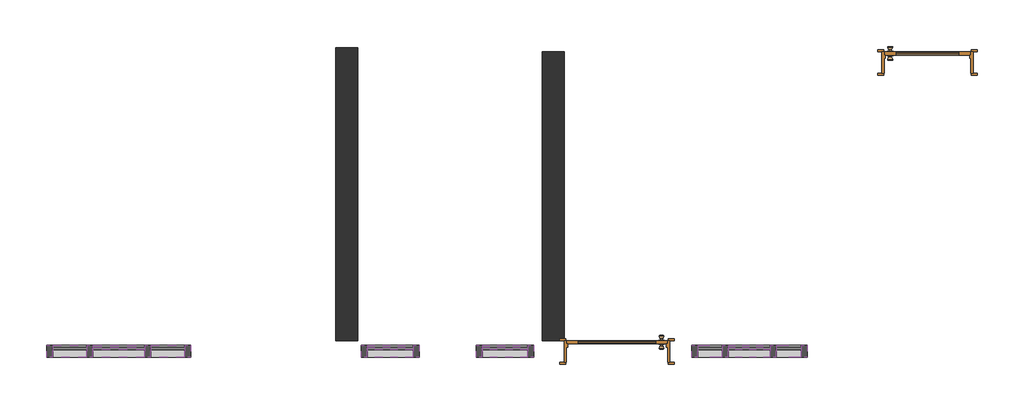
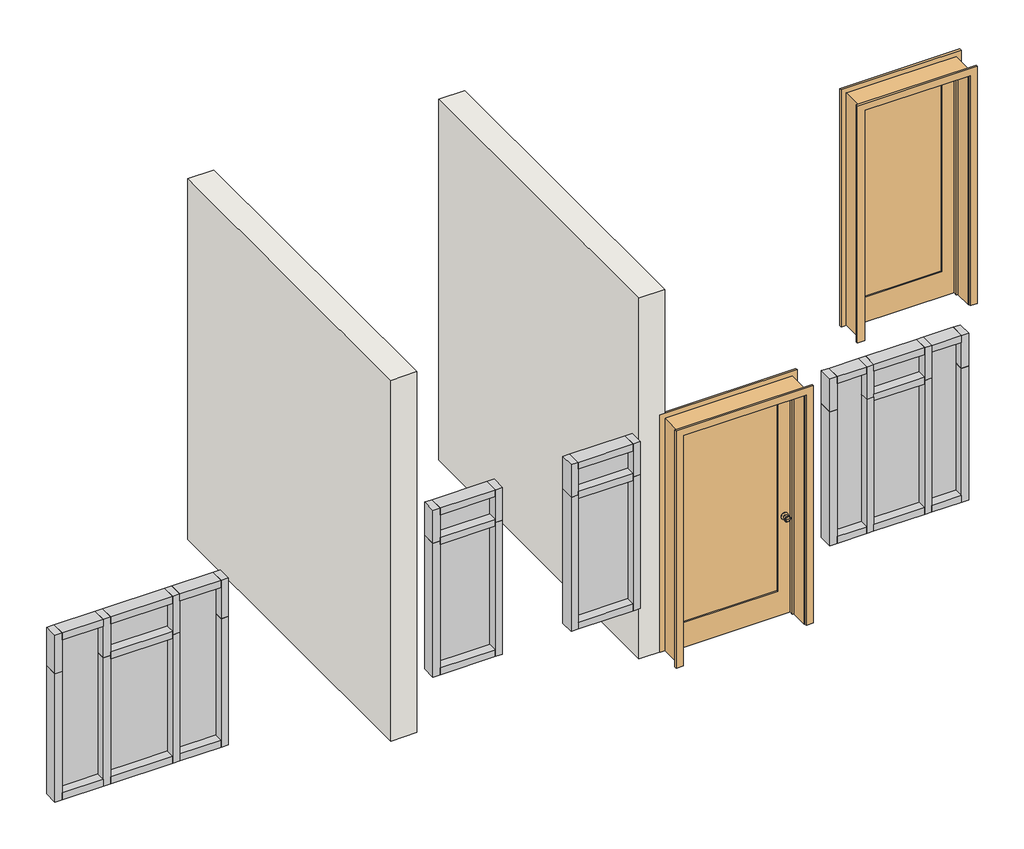
# One storey: 44 members, 12 plates, 2 doors, 2 walls.
"""IFC4 building model written with IfcOpenShell, lengths in millimetres."""

from ifc_helpers import new_model, si_unit, frame, origin, place, context, project, spatial, polyline, outline, extrude, faceted_brep, transform, mapped, element, save
from components import door_interior_single_1_panel_wood_3_x_7_3b97b8e7, door_0f538abb, member_86d06fe4, member_323df77c, member_71eb4692, member_843225dc, member_2d647432, member_0a1a1ade, member_a980948f, member_83167d3d, member_3c3dc66a, member_ca359333, member_ffcd2ccf, member_4adcbd6e, member_bc7dbe04, member_a1da5be3, member_718fe5d9, member_75d1e245, system_panel_glazed_030ff9b4, system_panel_glazed_82984963, system_panel_glazed_5eb04348, system_panel_glazed_05e747e2, system_panel_glazed_6bbf35ba, system_panel_glazed_1627a9b9, system_panel_glazed_6ade1748, system_panel_glazed_28683af0, system_panel_glazed_ad29da2a, system_panel_glazed_c196d27b

model = new_model("IFC4")

# Units and contexts
model_context = context("Model", 3, world=origin())
ifc_project = project(units=[si_unit("LENGTHUNIT", "METRE", prefix="MILLI")], contexts=[model_context])

# Site, building, storey
site = spatial("IfcSite", under=ifc_project)
building = spatial("IfcBuilding", under=site)
storey = spatial("IfcBuildingStorey", under=building, Elevation=609.6)

# Doors
placement = place(None, origin())
door_interior_single_1_panel_wood_3_x_7_shape = door_interior_single_1_panel_wood_3_x_7_3b97b8e7(model_context)
element("IfcDoor", 1, ObjectType="Door-Interior-Single-1_Panel-Wood : 3' x 7'", at=placement, inside=storey, context=model_context, shape_type="MappedRepresentation", body=[
    mapped(door_interior_single_1_panel_wood_3_x_7_shape, transform((6369.2850465, 1686.8408196, 609.6), x_axis=(1.0, 0.0, 0.0), y_axis=(0.0, 1.0, 0.0), z_axis=(0.0, 0.0, 1.0))),
])
door_shape = door_0f538abb(model_context)
element("IfcDoor", 2, ObjectType="Door-Interior-Single-1_Panel-Wood : 3'6\" x 7' DOOR", at=placement, inside=storey, context=model_context, shape_type="MappedRepresentation", body=[
    mapped(door_shape, transform((3092.6850465, -1361.1591804, 609.6), x_axis=(-1.0, 0.0, 0.0), y_axis=(0.0, -1.0, 0.0), z_axis=(0.0, 0.0, 1.0))),
])

# Members
member_shape = member_86d06fe4(model_context)
element("IfcMember", 3, ObjectType="Rectangular Mullion : 2.5\" x 5\" rectangular", at=placement, inside=storey, context=model_context, shape_type="MappedRepresentation", body=[
    mapped(member_shape, transform((940.0350465, -1364.3341804, 2768.6), x_axis=(0.0, 0.0, 1.0), y_axis=(0.0, -1.0, 0.0), z_axis=(1.0, 0.0, 0.0))),
])
element("IfcMember", 4, ObjectType="Rectangular Mullion : 2.5\" x 5\" rectangular", at=placement, inside=storey, context=model_context, shape_type="MappedRepresentation", body=[
    mapped(member_shape, transform((457.4350465, -1364.3341804, 1219.2), x_axis=(0.0, 0.0, -1.0), y_axis=(0.0, -1.0, 0.0), z_axis=(-1.0, 0.0, 0.0))),
])
member_2_shape = member_323df77c(model_context)
element("IfcMember", 5, ObjectType="Rectangular Mullion : 2.5\" x 5\" rectangular", at=placement, inside=storey, context=model_context, shape_type="MappedRepresentation", body=[
    mapped(member_2_shape, transform((940.0350465, -1364.3341804, 2463.8), x_axis=(0.0, 0.0, 1.0), y_axis=(0.0, -1.0, 0.0), z_axis=(1.0, 0.0, 0.0))),
])
member_3_shape = member_71eb4692(model_context)
element("IfcMember", 6, ObjectType="Rectangular Mullion : 2.5\" x 5\" rectangular", at=placement, inside=storey, context=model_context, shape_type="MappedRepresentation", body=[
    mapped(member_3_shape, transform((1003.5350465, -1364.3341804, 1219.2), x_axis=(1.0, 0.0, 0.0), y_axis=(0.0, -1.0, 0.0), z_axis=(0.0, 0.0, -1.0))),
])
element("IfcMember", 7, ObjectType="Rectangular Mullion : 2.5\" x 5\" rectangular", at=placement, inside=storey, context=model_context, shape_type="MappedRepresentation", body=[
    mapped(member_3_shape, transform((393.9350465, -1364.3341804, 2463.8), x_axis=(-1.0, 0.0, 0.0), y_axis=(0.0, -1.0, 0.0), z_axis=(0.0, 0.0, 1.0))),
])
element("IfcMember", 8, ObjectType="Rectangular Mullion : 2.5\" x 5\" rectangular", at=placement, inside=storey, context=model_context, shape_type="MappedRepresentation", body=[
    mapped(member_shape, transform((1670.2850465, -1364.3341804, 2768.6), x_axis=(0.0, 0.0, 1.0), y_axis=(0.0, 1.0, 0.0), z_axis=(-1.0, 0.0, 0.0))),
])
element("IfcMember", 9, ObjectType="Rectangular Mullion : 2.5\" x 5\" rectangular", at=placement, inside=storey, context=model_context, shape_type="MappedRepresentation", body=[
    mapped(member_shape, transform((2152.8850465, -1364.3341804, 1219.2), x_axis=(0.0, 0.0, -1.0), y_axis=(0.0, 1.0, 0.0), z_axis=(1.0, 0.0, 0.0))),
])
element("IfcMember", 10, ObjectType="Rectangular Mullion : 2.5\" x 5\" rectangular", at=placement, inside=storey, context=model_context, shape_type="MappedRepresentation", body=[
    mapped(member_2_shape, transform((1670.2850465, -1364.3341804, 2463.8), x_axis=(0.0, 0.0, 1.0), y_axis=(0.0, 1.0, 0.0), z_axis=(-1.0, 0.0, 0.0))),
])
element("IfcMember", 11, ObjectType="Rectangular Mullion : 2.5\" x 5\" rectangular", at=placement, inside=storey, context=model_context, shape_type="MappedRepresentation", body=[
    mapped(member_3_shape, transform((1606.7850465, -1364.3341804, 1219.2), x_axis=(-1.0, 0.0, 0.0), y_axis=(0.0, 1.0, 0.0), z_axis=(0.0, 0.0, -1.0))),
])
element("IfcMember", 12, ObjectType="Rectangular Mullion : 2.5\" x 5\" rectangular", at=placement, inside=storey, context=model_context, shape_type="MappedRepresentation", body=[
    mapped(member_3_shape, transform((2216.3850465, -1364.3341804, 2463.8), x_axis=(1.0, 0.0, 0.0), y_axis=(0.0, 1.0, 0.0), z_axis=(0.0, 0.0, 1.0))),
])
member_4_shape = member_843225dc(model_context)
element("IfcMember", 13, ObjectType="Rectangular Mullion : 2.5\" x 5\" rectangular", at=placement, inside=storey, context=model_context, shape_type="MappedRepresentation", body=[
    mapped(member_4_shape, transform((-1466.6149535, -1364.3341804, 2768.6), x_axis=(0.0, 0.0, 1.0), y_axis=(0.0, -1.0, 0.0), z_axis=(1.0, 0.0, 0.0))),
])
element("IfcMember", 14, ObjectType="Rectangular Mullion : 2.5\" x 5\" rectangular", at=placement, inside=storey, context=model_context, shape_type="MappedRepresentation", body=[
    mapped(member_4_shape, transform((-2501.6649535, -1364.3341804, 2768.6), x_axis=(0.0, 0.0, 1.0), y_axis=(0.0, -1.0, 0.0), z_axis=(1.0, 0.0, 0.0))),
])
element("IfcMember", 15, ObjectType="Rectangular Mullion : 2.5\" x 5\" rectangular", at=placement, inside=storey, context=model_context, shape_type="MappedRepresentation", body=[
    mapped(member_4_shape, transform((-2863.6149535, -1364.3341804, 1219.2), x_axis=(0.0, 0.0, -1.0), y_axis=(0.0, -1.0, 0.0), z_axis=(-1.0, 0.0, 0.0))),
])
element("IfcMember", 16, ObjectType="Rectangular Mullion : 2.5\" x 5\" rectangular", at=placement, inside=storey, context=model_context, shape_type="MappedRepresentation", body=[
    mapped(member_4_shape, transform((-1828.5649535, -1364.3341804, 1219.2), x_axis=(0.0, 0.0, -1.0), y_axis=(0.0, -1.0, 0.0), z_axis=(-1.0, 0.0, 0.0))),
])
member_5_shape = member_2d647432(model_context)
element("IfcMember", 17, ObjectType="Rectangular Mullion : 2.5\" x 5\" rectangular", at=placement, inside=storey, context=model_context, shape_type="MappedRepresentation", body=[
    mapped(member_5_shape, transform((-2469.9149535, -1364.3341804, 1219.2), x_axis=(1.0, 0.0, 0.0), y_axis=(0.0, -1.0, 0.0), z_axis=(0.0, 0.0, -1.0))),
])
element("IfcMember", 18, ObjectType="Rectangular Mullion : 2.5\" x 5\" rectangular", at=placement, inside=storey, context=model_context, shape_type="MappedRepresentation", body=[
    mapped(member_5_shape, transform((-1860.3149535, -1364.3341804, 1219.2), x_axis=(1.0, 0.0, 0.0), y_axis=(0.0, -1.0, 0.0), z_axis=(0.0, 0.0, -1.0))),
])
member_6_shape = member_0a1a1ade(model_context)
element("IfcMember", 19, ObjectType="Rectangular Mullion : 2.5\" x 5\" rectangular", at=placement, inside=storey, context=model_context, shape_type="MappedRepresentation", body=[
    mapped(member_6_shape, transform((-1892.0649535, -1364.3341804, 2413.0), x_axis=(0.0, 0.0, 1.0), y_axis=(0.0, -1.0, 0.0), z_axis=(1.0, 0.0, 0.0))),
])
member_7_shape = member_a980948f(model_context)
element("IfcMember", 20, ObjectType="Rectangular Mullion : 2.5\" x 5\" rectangular", at=placement, inside=storey, context=model_context, shape_type="MappedRepresentation", body=[
    mapped(member_7_shape, transform((-2438.1649535, -1364.3341804, 1219.2), x_axis=(0.0, 0.0, -1.0), y_axis=(0.0, -1.0, 0.0), z_axis=(-1.0, 0.0, 0.0))),
])
element("IfcMember", 21, ObjectType="Rectangular Mullion : 2.5\" x 5\" rectangular", at=placement, inside=storey, context=model_context, shape_type="MappedRepresentation", body=[
    mapped(member_7_shape, transform((-1892.0649535, -1364.3341804, 2768.6), x_axis=(0.0, 0.0, 1.0), y_axis=(0.0, -1.0, 0.0), z_axis=(1.0, 0.0, 0.0))),
])
member_8_shape = member_83167d3d(model_context)
element("IfcMember", 22, ObjectType="Rectangular Mullion : 2.5\" x 5\" rectangular", at=placement, inside=storey, context=model_context, shape_type="MappedRepresentation", body=[
    mapped(member_8_shape, transform((-1403.1149535, -1364.3341804, 1219.2), x_axis=(1.0, 0.0, 0.0), y_axis=(0.0, -1.0, 0.0), z_axis=(0.0, 0.0, -1.0))),
])
element("IfcMember", 23, ObjectType="Rectangular Mullion : 2.5\" x 5\" rectangular", at=placement, inside=storey, context=model_context, shape_type="MappedRepresentation", body=[
    mapped(member_8_shape, transform((-2927.1149535, -1364.3341804, 2413.0), x_axis=(-1.0, 0.0, 0.0), y_axis=(0.0, -1.0, 0.0), z_axis=(0.0, 0.0, 1.0))),
])
member_9_shape = member_3c3dc66a(model_context)
element("IfcMember", 24, ObjectType="Rectangular Mullion : 2.5\" x 5\" rectangular", at=placement, inside=storey, context=model_context, shape_type="MappedRepresentation", body=[
    mapped(member_9_shape, transform((2216.3850465, -1364.3341804, 2768.6), x_axis=(1.0, 0.0, 0.0), y_axis=(0.0, 1.0, 0.0), z_axis=(0.0, 0.0, 1.0))),
])
element("IfcMember", 25, ObjectType="Rectangular Mullion : 2.5\" x 5\" rectangular", at=placement, inside=storey, context=model_context, shape_type="MappedRepresentation", body=[
    mapped(member_9_shape, transform((1606.7850465, -1364.3341804, 2463.8), x_axis=(-1.0, 0.0, 0.0), y_axis=(0.0, 1.0, 0.0), z_axis=(0.0, 0.0, -1.0))),
])
element("IfcMember", 26, ObjectType="Rectangular Mullion : 2.5\" x 5\" rectangular", at=placement, inside=storey, context=model_context, shape_type="MappedRepresentation", body=[
    mapped(member_9_shape, transform((393.9350465, -1364.3341804, 2768.6), x_axis=(-1.0, 0.0, 0.0), y_axis=(0.0, -1.0, 0.0), z_axis=(0.0, 0.0, 1.0))),
])
element("IfcMember", 27, ObjectType="Rectangular Mullion : 2.5\" x 5\" rectangular", at=placement, inside=storey, context=model_context, shape_type="MappedRepresentation", body=[
    mapped(member_9_shape, transform((1003.5350465, -1364.3341804, 2463.8), x_axis=(1.0, 0.0, 0.0), y_axis=(0.0, -1.0, 0.0), z_axis=(0.0, 0.0, -1.0))),
])
member_10_shape = member_ca359333(model_context)
element("IfcMember", 28, ObjectType="Rectangular Mullion : 2.5\" x 5\" rectangular", at=placement, inside=storey, context=model_context, shape_type="MappedRepresentation", body=[
    mapped(member_10_shape, transform((-2469.9149535, -1364.3341804, 2413.0), x_axis=(1.0, 0.0, 0.0), y_axis=(0.0, -1.0, 0.0), z_axis=(0.0, 0.0, -1.0))),
])
element("IfcMember", 29, ObjectType="Rectangular Mullion : 2.5\" x 5\" rectangular", at=placement, inside=storey, context=model_context, shape_type="MappedRepresentation", body=[
    mapped(member_10_shape, transform((-1860.3149535, -1364.3341804, 2413.0), x_axis=(1.0, 0.0, 0.0), y_axis=(0.0, -1.0, 0.0), z_axis=(0.0, 0.0, -1.0))),
])
member_11_shape = member_ffcd2ccf(model_context)
element("IfcMember", 30, ObjectType="Rectangular Mullion : 2.5\" x 5\" rectangular", at=placement, inside=storey, context=model_context, shape_type="MappedRepresentation", body=[
    mapped(member_11_shape, transform((-2927.1149535, -1364.3341804, 2768.6), x_axis=(-1.0, 0.0, 0.0), y_axis=(0.0, -1.0, 0.0), z_axis=(0.0, 0.0, 1.0))),
])
element("IfcMember", 31, ObjectType="Rectangular Mullion : 2.5\" x 5\" rectangular", at=placement, inside=storey, context=model_context, shape_type="MappedRepresentation", body=[
    mapped(member_11_shape, transform((-1403.1149535, -1364.3341804, 2413.0), x_axis=(1.0, 0.0, 0.0), y_axis=(0.0, -1.0, 0.0), z_axis=(0.0, 0.0, -1.0))),
])
element("IfcMember", 32, ObjectType="Rectangular Mullion : 2.5\" x 5\" rectangular", at=placement, inside=storey, context=model_context, shape_type="MappedRepresentation", body=[
    mapped(member_9_shape, transform((3880.0850465, -1364.3341804, 2768.6), x_axis=(-1.0, 0.0, 0.0), y_axis=(0.0, -1.0, 0.0), z_axis=(0.0, 0.0, 1.0))),
])
element("IfcMember", 33, ObjectType="Rectangular Mullion : 2.5\" x 5\" rectangular", at=placement, inside=storey, context=model_context, shape_type="MappedRepresentation", body=[
    mapped(member_3_shape, transform((5099.2850465, -1364.3341804, 1219.2), x_axis=(1.0, 0.0, 0.0), y_axis=(0.0, -1.0, 0.0), z_axis=(0.0, 0.0, -1.0))),
])
element("IfcMember", 34, ObjectType="Rectangular Mullion : 2.5\" x 5\" rectangular", at=placement, inside=storey, context=model_context, shape_type="MappedRepresentation", body=[
    mapped(member_9_shape, transform((5099.2850465, -1364.3341804, 2463.8), x_axis=(1.0, 0.0, 0.0), y_axis=(0.0, -1.0, 0.0), z_axis=(0.0, 0.0, -1.0))),
])
element("IfcMember", 35, ObjectType="Rectangular Mullion : 2.5\" x 5\" rectangular", at=placement, inside=storey, context=model_context, shape_type="MappedRepresentation", body=[
    mapped(member_3_shape, transform((3880.0850465, -1364.3341804, 2463.8), x_axis=(-1.0, 0.0, 0.0), y_axis=(0.0, -1.0, 0.0), z_axis=(0.0, 0.0, 1.0))),
])
member_12_shape = member_4adcbd6e(model_context)
element("IfcMember", 36, ObjectType="Rectangular Mullion : 2.5\" x 5\" rectangular", at=placement, inside=storey, context=model_context, shape_type="MappedRepresentation", body=[
    mapped(member_12_shape, transform((5035.7850465, -1364.3341804, 2768.6), x_axis=(0.0, 0.0, 1.0), y_axis=(0.0, -1.0, 0.0), z_axis=(1.0, 0.0, 0.0))),
])
element("IfcMember", 37, ObjectType="Rectangular Mullion : 2.5\" x 5\" rectangular", at=placement, inside=storey, context=model_context, shape_type="MappedRepresentation", body=[
    mapped(member_12_shape, transform((4203.9350465, -1364.3341804, 2768.6), x_axis=(0.0, 0.0, 1.0), y_axis=(0.0, -1.0, 0.0), z_axis=(1.0, 0.0, 0.0))),
])
element("IfcMember", 38, ObjectType="Rectangular Mullion : 2.5\" x 5\" rectangular", at=placement, inside=storey, context=model_context, shape_type="MappedRepresentation", body=[
    mapped(member_12_shape, transform((3943.5850465, -1364.3341804, 1219.2), x_axis=(0.0, 0.0, -1.0), y_axis=(0.0, -1.0, 0.0), z_axis=(-1.0, 0.0, 0.0))),
])
element("IfcMember", 39, ObjectType="Rectangular Mullion : 2.5\" x 5\" rectangular", at=placement, inside=storey, context=model_context, shape_type="MappedRepresentation", body=[
    mapped(member_12_shape, transform((4775.4350465, -1364.3341804, 1219.2), x_axis=(0.0, 0.0, -1.0), y_axis=(0.0, -1.0, 0.0), z_axis=(-1.0, 0.0, 0.0))),
])
member_13_shape = member_bc7dbe04(model_context)
element("IfcMember", 40, ObjectType="Rectangular Mullion : 2.5\" x 5\" rectangular", at=placement, inside=storey, context=model_context, shape_type="MappedRepresentation", body=[
    mapped(member_13_shape, transform((4267.4350465, -1364.3341804, 1219.2), x_axis=(0.0, 0.0, -1.0), y_axis=(0.0, -1.0, 0.0), z_axis=(-1.0, 0.0, 0.0))),
])
element("IfcMember", 41, ObjectType="Rectangular Mullion : 2.5\" x 5\" rectangular", at=placement, inside=storey, context=model_context, shape_type="MappedRepresentation", body=[
    mapped(member_13_shape, transform((4711.9350465, -1364.3341804, 2768.6), x_axis=(0.0, 0.0, 1.0), y_axis=(0.0, -1.0, 0.0), z_axis=(1.0, 0.0, 0.0))),
])
member_14_shape = member_a1da5be3(model_context)
element("IfcMember", 42, ObjectType="Rectangular Mullion : 2.5\" x 5\" rectangular", at=placement, inside=storey, context=model_context, shape_type="MappedRepresentation", body=[
    mapped(member_14_shape, transform((4235.6850465, -1364.3341804, 1219.2), x_axis=(1.0, 0.0, 0.0), y_axis=(0.0, -1.0, 0.0), z_axis=(0.0, 0.0, -1.0))),
])
element("IfcMember", 43, ObjectType="Rectangular Mullion : 2.5\" x 5\" rectangular", at=placement, inside=storey, context=model_context, shape_type="MappedRepresentation", body=[
    mapped(member_14_shape, transform((4743.6850465, -1364.3341804, 1219.2), x_axis=(1.0, 0.0, 0.0), y_axis=(0.0, -1.0, 0.0), z_axis=(0.0, 0.0, -1.0))),
])
member_15_shape = member_718fe5d9(model_context)
element("IfcMember", 44, ObjectType="Rectangular Mullion : 2.5\" x 5\" rectangular", at=placement, inside=storey, context=model_context, shape_type="MappedRepresentation", body=[
    mapped(member_15_shape, transform((4711.9350465, -1364.3341804, 2463.8), x_axis=(0.0, 0.0, 1.0), y_axis=(0.0, -1.0, 0.0), z_axis=(1.0, 0.0, 0.0))),
])
member_16_shape = member_75d1e245(model_context)
element("IfcMember", 45, ObjectType="Rectangular Mullion : 2.5\" x 5\" rectangular", at=placement, inside=storey, context=model_context, shape_type="MappedRepresentation", body=[
    mapped(member_16_shape, transform((4235.6850465, -1364.3341804, 2463.8), x_axis=(1.0, 0.0, 0.0), y_axis=(0.0, -1.0, 0.0), z_axis=(0.0, 0.0, -1.0))),
])
element("IfcMember", 46, ObjectType="Rectangular Mullion : 2.5\" x 5\" rectangular", at=placement, inside=storey, context=model_context, shape_type="MappedRepresentation", body=[
    mapped(member_16_shape, transform((4743.6850465, -1364.3341804, 2463.8), x_axis=(1.0, 0.0, 0.0), y_axis=(0.0, -1.0, 0.0), z_axis=(0.0, 0.0, -1.0))),
])

# Plates
system_panel_glazed_shape = system_panel_glazed_030ff9b4(model_context)
element("IfcPlate", 47, ObjectType="System Panel : Glazed", at=placement, inside=storey, context=model_context, shape_type="MappedRepresentation", body=[
    mapped(system_panel_glazed_shape, transform((698.7350465, -1364.3341804, 1282.7), x_axis=(1.0, 0.0, 0.0), y_axis=(0.0, 1.0, 0.0), z_axis=(0.0, 0.0, 1.0))),
])
system_panel_glazed_2_shape = system_panel_glazed_82984963(model_context)
element("IfcPlate", 48, ObjectType="System Panel : Glazed", at=placement, inside=storey, context=model_context, shape_type="MappedRepresentation", body=[
    mapped(system_panel_glazed_2_shape, transform((1911.5850465, -1364.3341804, 1282.7), x_axis=(-1.0, 0.0, 0.0), y_axis=(0.0, -1.0, 0.0), z_axis=(0.0, 0.0, 1.0))),
])
system_panel_glazed_3_shape = system_panel_glazed_5eb04348(model_context)
element("IfcPlate", 49, ObjectType="System Panel : Glazed", at=placement, inside=storey, context=model_context, shape_type="MappedRepresentation", body=[
    mapped(system_panel_glazed_3_shape, transform((-2165.1149535, -1364.3341804, 1282.7), x_axis=(1.0, 0.0, 0.0), y_axis=(0.0, 1.0, 0.0), z_axis=(0.0, 0.0, 1.0))),
])
system_panel_glazed_4_shape = system_panel_glazed_05e747e2(model_context)
element("IfcPlate", 50, ObjectType="System Panel : Glazed", at=placement, inside=storey, context=model_context, shape_type="MappedRepresentation", body=[
    mapped(system_panel_glazed_4_shape, transform((1911.5850465, -1364.3341804, 2495.55), x_axis=(-1.0, 0.0, 0.0), y_axis=(0.0, -1.0, 0.0), z_axis=(0.0, 0.0, 1.0))),
])
system_panel_glazed_5_shape = system_panel_glazed_6bbf35ba(model_context)
element("IfcPlate", 51, ObjectType="System Panel : Glazed", at=placement, inside=storey, context=model_context, shape_type="MappedRepresentation", body=[
    mapped(system_panel_glazed_5_shape, transform((698.7350465, -1364.3341804, 2495.55), x_axis=(1.0, 0.0, 0.0), y_axis=(0.0, 1.0, 0.0), z_axis=(0.0, 0.0, 1.0))),
])
system_panel_glazed_6_shape = system_panel_glazed_1627a9b9(model_context)
element("IfcPlate", 52, ObjectType="System Panel : Glazed", at=placement, inside=storey, context=model_context, shape_type="MappedRepresentation", body=[
    mapped(system_panel_glazed_6_shape, transform((-2682.6399535, -1364.3341804, 1282.7), x_axis=(1.0, 0.0, 0.0), y_axis=(0.0, 1.0, 0.0), z_axis=(0.0, 0.0, 1.0))),
])
element("IfcPlate", 53, ObjectType="System Panel : Glazed", at=placement, inside=storey, context=model_context, shape_type="MappedRepresentation", body=[
    mapped(system_panel_glazed_6_shape, transform((-1647.5899535, -1364.3341804, 1282.7), x_axis=(1.0, 0.0, 0.0), y_axis=(0.0, 1.0, 0.0), z_axis=(0.0, 0.0, 1.0))),
])
system_panel_glazed_7_shape = system_panel_glazed_6ade1748(model_context)
element("IfcPlate", 54, ObjectType="System Panel : Glazed", at=placement, inside=storey, context=model_context, shape_type="MappedRepresentation", body=[
    mapped(system_panel_glazed_7_shape, transform((-2165.1149535, -1364.3341804, 2444.75), x_axis=(1.0, 0.0, 0.0), y_axis=(0.0, 1.0, 0.0), z_axis=(0.0, 0.0, 1.0))),
])
system_panel_glazed_8_shape = system_panel_glazed_28683af0(model_context)
element("IfcPlate", 55, ObjectType="System Panel : Glazed", at=placement, inside=storey, context=model_context, shape_type="MappedRepresentation", body=[
    mapped(system_panel_glazed_8_shape, transform((4073.7600465, -1364.3341804, 1282.7), x_axis=(1.0, 0.0, 0.0), y_axis=(0.0, 1.0, 0.0), z_axis=(0.0, 0.0, 1.0))),
])
element("IfcPlate", 56, ObjectType="System Panel : Glazed", at=placement, inside=storey, context=model_context, shape_type="MappedRepresentation", body=[
    mapped(system_panel_glazed_8_shape, transform((4905.6100465, -1364.3341804, 1282.7), x_axis=(1.0, 0.0, 0.0), y_axis=(0.0, 1.0, 0.0), z_axis=(0.0, 0.0, 1.0))),
])
system_panel_glazed_9_shape = system_panel_glazed_ad29da2a(model_context)
element("IfcPlate", 57, ObjectType="System Panel : Glazed", at=placement, inside=storey, context=model_context, shape_type="MappedRepresentation", body=[
    mapped(system_panel_glazed_9_shape, transform((4489.6850465, -1364.3341804, 1282.7), x_axis=(1.0, 0.0, 0.0), y_axis=(0.0, 1.0, 0.0), z_axis=(0.0, 0.0, 1.0))),
])
system_panel_glazed_10_shape = system_panel_glazed_c196d27b(model_context)
element("IfcPlate", 58, ObjectType="System Panel : Glazed", at=placement, inside=storey, context=model_context, shape_type="MappedRepresentation", body=[
    mapped(system_panel_glazed_10_shape, transform((4489.6850465, -1364.3341804, 2495.55), x_axis=(1.0, 0.0, 0.0), y_axis=(0.0, 1.0, 0.0), z_axis=(0.0, 0.0, 1.0))),
])

# Walls
element("IfcWall", 59, ObjectType="9\" wall", at=placement, inside=storey, context=model_context, shape_type="Brep", body=[
    faceted_brep([(2533.8850465, -1250.0341804, 3962.4), (2533.8850465, -1250.0341804, 3810.0), (2533.8850465, -1250.0341804, 2768.6), (2533.8850465, -1250.0341804, 609.6), (2533.8850465, 1797.9658196, 609.6), (2533.8850465, 1797.9658196, 3962.4), (2305.2850465, -1250.0341804, 609.6), (2305.2850465, -1250.0341804, 3962.4), (2305.2850465, 1797.9658196, 3962.4), (2305.2850465, 1797.9658196, 609.6)], [[[0, 1, 2, 3, 4, 5]], [[6, 7, 8, 9]], [[4, 3, 6, 9]], [[5, 4, 9, 8]], [[0, 5, 8, 7]], [[0, 7, 6, 3, 2, 1]]]),
])
element("IfcWall", 60, ObjectType="9\" wall", at=placement, inside=storey, context=model_context, shape_type="SweptSolid", body=[
    extrude(outline(polyline([(355.8350465, 1839.2408196), (355.8350465, -1250.0341804), (127.2350465, -1250.0341804), (127.2350465, 1839.2408196), (355.8350465, 1839.2408196)])), frame((0.0, 0.0, 609.6), z_axis=(0.0, 0.0, 1.0), x_axis=(1.0, 0.0, 0.0)), (0.0, 0.0, 1.0), 3352.8),
])

save(model, "model.ifc")

# Revit data of these elements
# Type "Door-Interior-Single-1_Panel-Wood : 3' x 7'"
#   Type Mark = "10"
#   Assembly Code = "C1020300"
#   Analytic Construction = "Wooden"
#   Top Rail = 0' - 4 11/16"
#   Thickness = 0' - 1 3/8"
#   Thermal Resistance (R) = 2.5876 (h·ft²·°F)/BTU
#   Swing Angle [instance default] = 90.00°
#   Stiles = 0' - 4 3/4"
#   Rough Width = 3' - 2"
#   Rough Height = 7' - 1"
#   Height = 7' - 0"
#   Width = 3' - 0"
#   Heat Transfer Coefficient (U) = 0.3865 BTU/(h·ft²·°F)
#   Bottom Rail = 0' - 9 1/8"
#   Trim Material = DOOR 3'6" X 7'
#   Panel Material = DOOR 3'6" X 7'
#   Frame Material = DOOR 3'6" X 7'
#   Door Handle Material = Aluminum
#   Visual Light Transmittance = 0
#   Solar Heat Gain Coefficient = 0
#   Wall Closure = (empty or 0)
#   Function = (empty or 0)
# Type "Door-Interior-Single-1_Panel-Wood : 3'6\" x 7' DOOR"
#   Type Mark = "9"
#   Assembly Code = "C1020300"
#   Analytic Construction = "Wooden"
#   Top Rail = 0' - 4 11/16"
#   Thickness = 0' - 1 3/8"
#   Thermal Resistance (R) = 2.5876 (h·ft²·°F)/BTU
#   Swing Angle [instance default] = 90.00°
#   Stiles = 0' - 4 3/4"
#   Rough Width = 3' - 8"
#   Rough Height = 7' - 1"
#   Height = 7' - 0"
#   Width = 3' - 6"
#   Heat Transfer Coefficient (U) = 0.3865 BTU/(h·ft²·°F)
#   Bottom Rail = 0' - 9 1/8"
#   Trim Material = DOOR 3'6" X 7'
#   Panel Material = DOOR 3'6" X 7'
#   Frame Material = DOOR 3'6" X 7'
#   Door Handle Material = Aluminum
#   Visual Light Transmittance = 0
#   Solar Heat Gain Coefficient = 0
#   Wall Closure = (empty or 0)
#   Function = (empty or 0)
# Type "Rectangular Mullion : 2.5\" x 5\" rectangular"
#   built-in parameter 1007304 = 0.416667 (stored number, unit not read)
#   built-in parameter 1007301 = 0.104167 (stored number, unit not read)
#   built-in parameter 1007300 = 0.104167 (stored number, unit not read)
# Type "System Panel : Glazed"
#   Construction Type Id = "GSP4R"
#   Analytic Construction = "1/8 in Pilkington single glazing"
#   Visual Light Transmittance = 0.9
#   Solar Heat Gain Coefficient = 0.86
#   Heat Transfer Coefficient (U) = 1.18115 BTU/(h·ft²·°F)
#   Define Thermal Properties by = 1
# Type "9\" wall"
#   Assembly Code = "B2010"
#   Layers, outside or top first: 0' - 9" no material (function 1)
# Element 1 (IfcDoor, "Door-Interior-Single-1_Panel-Wood : 3' x 7'")
#   Swing Angle = 90.00°
#   Phase Created = New Construction
#   Materials on its faces: "DOOR 3'6\" X 7'", "Aluminum"
# Element 2 (IfcDoor, "Door-Interior-Single-1_Panel-Wood : 3'6\" x 7' DOOR")
#   Swing Angle = 90.00°
#   Phase Created = New Construction
#   Materials on its faces: "DOOR 3'6\" X 7'", "Aluminum"
# Elements 3, 4, 5, 6, 7, 8, 9, 10, 11, 12, 13, 14, 15, 16, 17, 18, 19, 20, 21, 22, 23, 24, 25, 26, 27, 28, 29, 30, 31, 32, 33, 34, 35, 36, 37, 38, 39, 40, 41, 42, 43, 44, 45, 46 (IfcMember, "Rectangular Mullion : 2.5\" x 5\" rectangular")
#   Phase Created = New Construction
# Elements 47, 48, 49, 50, 51, 52, 53, 54, 55, 56, 57, 58 (IfcPlate, "System Panel : Glazed")
#   Phase Created = New Construction
#   Materials on its faces: "Glass"
# Elements 59, 60 (IfcWall, "9\" wall")
#   Top Offset = 0' - 0"
#   Base Offset = 0' - 0"
#   wall height = 11' - 0"
#   Phase Created = New Construction
#   Top Constraint = 3 SLAB
#   Materials on its faces: "Default Wall"
# Materials
#   "DOOR 3'6\" X 7'": class "Generic", colour RGB 120 120 120, transparency 0, Cost = 0
#   "Aluminum": class "Metal", colour RGB 247 247 247, transparency 0, Description = "Aluminum 6061", Cost = 0
#   "Glass": class "Glass", colour RGB 0 128 192, transparency 0.75, Description = "Soda Lime Glass", Cost = 0
#   "Default Wall": colour RGB 128 128 128, transparency 0, Cost = 0
